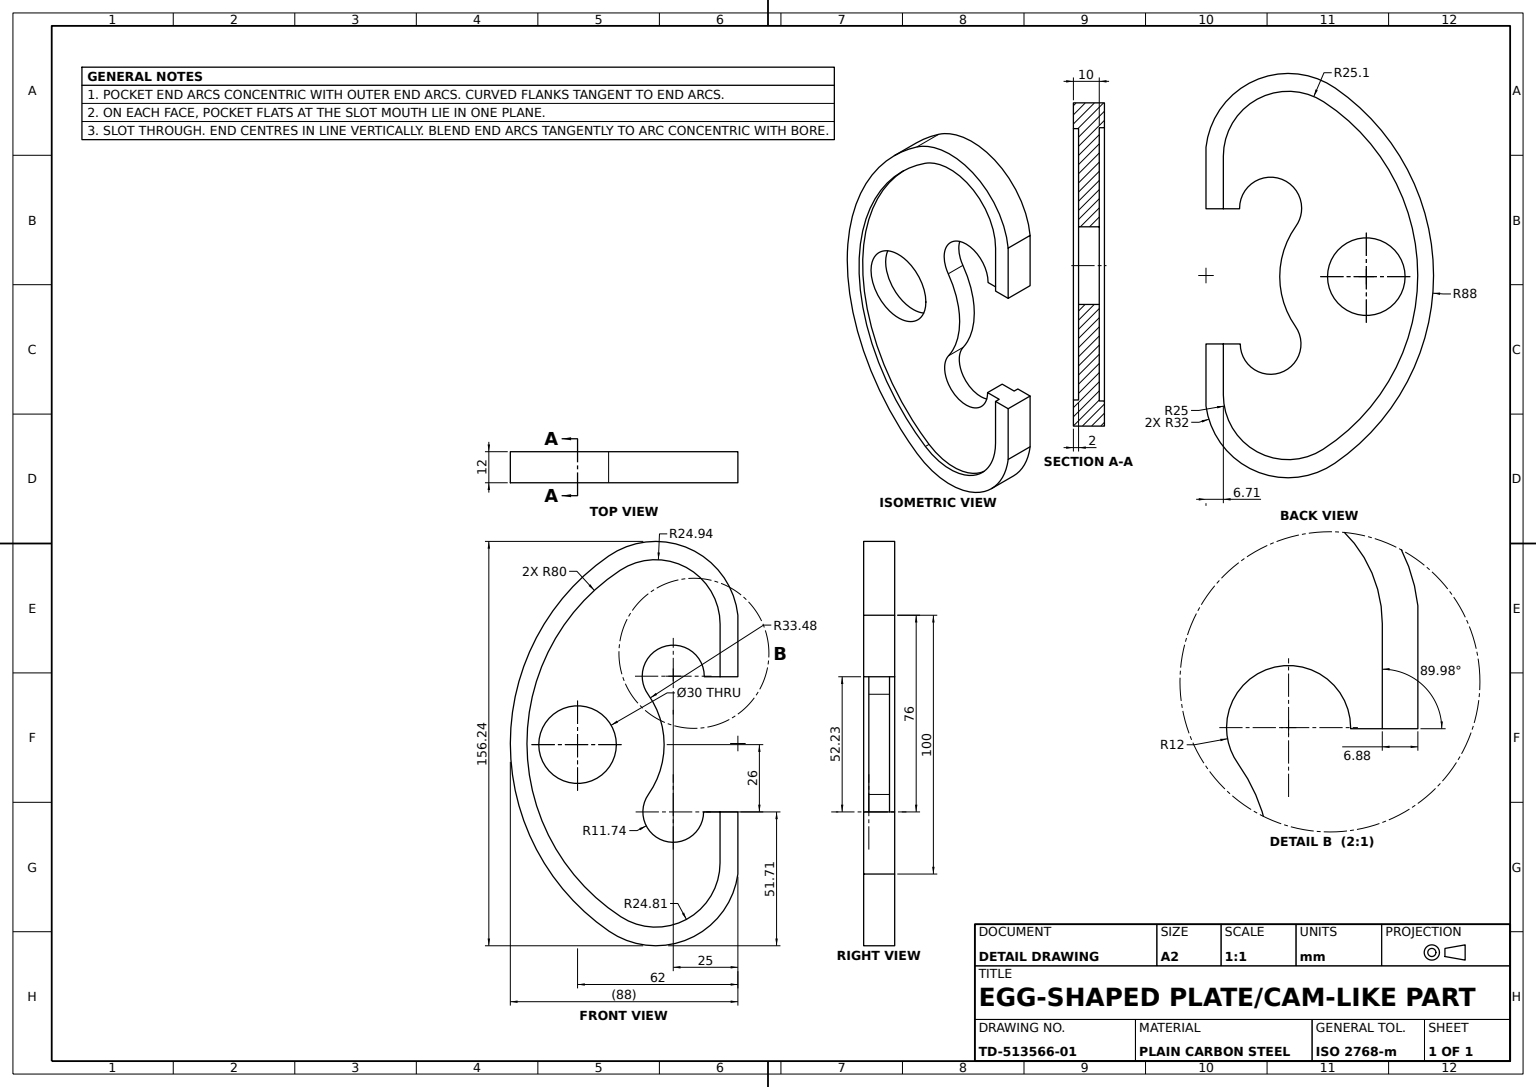
from build123d import *

# Parameters (mm, degrees)
PLATE_BODY_12MM_DEPTH   = 12
THROUGH_HOLE_SKETCH_R   = 15
THROUGH_HOLE_DEPTH      = 12
FACE_POCKET_A_2MM_DEPTH = 2
FACE_POCKET_B_2MM_DEPTH = 2
SLOT_OPENING_CUT_DEPTH  = 10
RIM_NOTCH_A_SKETCH_W    = 6.711695518
RIM_NOTCH_A_SKETCH_H    = 52.229672595
RIM_NOTCH_A_DEPTH       = 10
RIM_NOTCH_B_SKETCH_W    = 2
RIM_NOTCH_B_SKETCH_H    = 52.229672595
RIM_NOTCH_B_DEPTH       = 10


with BuildPart() as part:
    # Plate Outline Sketch → Plate Body 12mm (new body)
    with BuildSketch(Plane.XY):
        with BuildLine():
            Line((0, -76), (0, 0))
            Line((0, 0), (0, 11.558252986))
            ThreePointArc((0, 11.558252986), (-10.446142685, 31.91035387), (-31.811209757, 40.087383673))
            ThreePointArc((-31.811209757, 40.087383673), (-41.331169578, 38.638494373), (-49.989043904, 34.423031486))
            ThreePointArc((-49.989043904, 34.423031486), (-87.99994879, -38.094936415), (-49.832664385, -110.530721493))
            ThreePointArc((-49.832664385, -110.530721493), (-41.198690561, -114.717276949), (-31.711695518, -116.155913677))
            ThreePointArc((-31.711695518, -116.155913677), (-10.653997006, -108.251003081), (0, -88.441747014))
            Line((0, -88.441747014), (0, -76))
        make_face()
    extrude(amount=PLATE_BODY_12MM_DEPTH)

    # Through Hole Sketch → Through Hole (cut)
    with BuildSketch(Plane.XY.offset(12)):
        with Locations((-62, -38.441747014)):
            Circle(THROUGH_HOLE_SKETCH_R)
    extrude(amount=-THROUGH_HOLE_DEPTH, mode=Mode.SUBTRACT)

    # Face Pocket A Sketch → Face Pocket A 2mm (cut)
    with BuildSketch(Plane.XY.offset(12)):
        with BuildLine():
            Line((-6.873473723, 8.080280991), (-6.899746136, -84.162980533))
            ThreePointArc((-6.899746136, -84.162980533), (-19.89556251, -105.973610229), (-45.263391889, -104.940148269))
            ThreePointArc((-45.263391889, -104.940148269), (-81.569163873, -38.072577616), (-45.50779291, 28.927113491))
            ThreePointArc((-45.50779291, 28.927113491), (-19.968976613, 30.033960698), (-6.873473723, 8.080280991))
        make_face()
    extrude(amount=-FACE_POCKET_A_2MM_DEPTH, mode=Mode.SUBTRACT)

    # Face Pocket B Sketch → Face Pocket B 2mm (cut)
    with BuildSketch(Plane(origin=(0, 0, 0), x_dir=(-1, 0, 0), z_dir=(0, 0, -1))):
        with BuildLine():
            Line((6.711695518, 8.087383673), (6.711695518, -84.155913677))
            ThreePointArc((6.711695518, -84.155913677), (19.751029382, -106.109101728), (45.267092765, -105.161893908))
            ThreePointArc((45.267092765, -105.161893908), (81.889710646, -38.07598005), (45.490730045, 29.131535823))
            ThreePointArc((45.490730045, 29.131535823), (19.839653868, 30.147924569), (6.711695518, 8.087383673))
        make_face()
    extrude(amount=-FACE_POCKET_B_2MM_DEPTH, mode=Mode.SUBTRACT)

    # Slot Opening Sketch → Slot Opening Cut (cut)
    with BuildSketch(Plane.XY.offset(10)):
        with BuildLine():
            Line((-12.997971015, -12.212074419), (-6.879253323, -12.212074419))
            Line((-6.879253323, -12.212074419), (0, -12.212074419))
            Line((0, -12.212074419), (0, -64.441747014))
            Line((0, -64.441747014), (-6.894129201, -64.441747014))
            Line((-6.894129201, -64.441747014), (-13.258551293, -64.441747014))
            ThreePointArc((-13.258551293, -64.441747014), (-28.540083812, -75.636809513), (-34.606755841, -57.691053721))
            ThreePointArc((-34.606755841, -57.691053721), (-28.520033449, -38.309557921), (-34.759611769, -18.976730106))
            ThreePointArc((-34.759611769, -18.976730106), (-28.558192424, -0.540946638), (-12.997971015, -12.212074419))
        make_face()
    extrude(amount=-SLOT_OPENING_CUT_DEPTH, mode=Mode.SUBTRACT)

    # Rim Notch A Sketch → Rim Notch A (cut)
    with BuildSketch(Plane(origin=(0, 0, 10), x_dir=(-1, 0, 0), z_dir=(0, 0, -1))):
        with Locations((3.355847759, -38.326910717)):
            Rectangle(RIM_NOTCH_A_SKETCH_W, RIM_NOTCH_A_SKETCH_H)
    extrude(amount=-RIM_NOTCH_A_DEPTH, mode=Mode.SUBTRACT)

    # Rim Notch B Sketch → Rim Notch B (cut)
    with BuildSketch(Plane(origin=(-6.711695518, 0, 0), x_dir=(0, 0, -1), z_dir=(1, 0, 0))):
        with Locations((-11, -38.326910717)):
            Rectangle(RIM_NOTCH_B_SKETCH_W, RIM_NOTCH_B_SKETCH_H)
    extrude(amount=-RIM_NOTCH_B_DEPTH, mode=Mode.SUBTRACT)


solid = part.part
